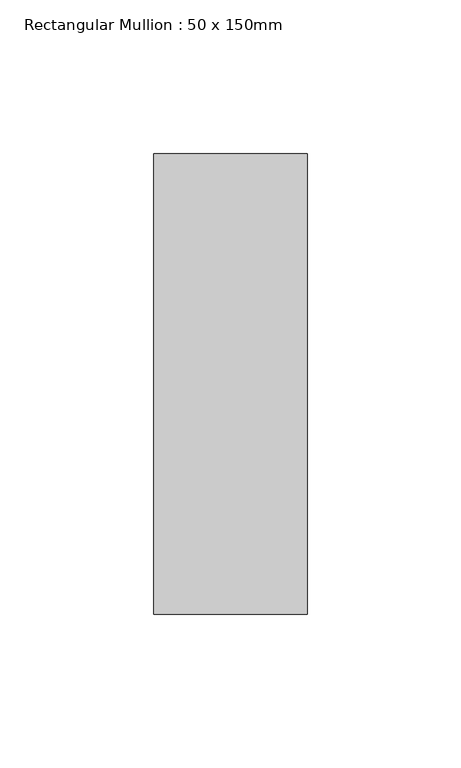
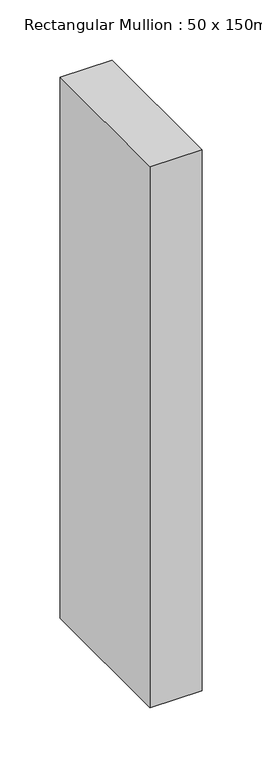
"""IFC4 building model written with IfcOpenShell, lengths in millimetres: member geometry, Rectangular Mullion : 50 x 150mm."""

from ifc_helpers import new_model, si_unit, frame, origin, place, context, project, spatial, polyline, outline, extrude, source, transform, mapped, element, save


def rectangular_mullion_50_x_150mm_5dbd0429(model_context):
    return source(origin(), model_context, "Body", "SweptSolid", [
        extrude(outline(polyline([(0.0, 75.0), (0.0, -75.0), (-50.0, -75.0), (-50.0, 75.0), (0.0, 75.0)])), frame((0.0, 0.0, -550.0), z_axis=(0.0, 0.0, 1.0), x_axis=(1.0, 0.0, 0.0)), (0.0, 0.0, 1.0), 550.0),
    ])


if __name__ == "__main__":
    model = new_model("IFC4")
    model_context = context("Model", 3, world=origin())
    ifc_project = project(units=[si_unit("LENGTHUNIT", "METRE", prefix="MILLI")], contexts=[model_context])
    site = spatial("IfcSite", under=ifc_project)
    building = spatial("IfcBuilding", under=site)
    placement = place(None, origin())
    rectangular_mullion_50_x_150mm_shape = rectangular_mullion_50_x_150mm_5dbd0429(model_context)
    element("IfcMember", 1, ObjectType="Rectangular Mullion : 50 x 150mm", at=placement, inside=building, context=model_context, shape_type="MappedRepresentation", body=[
        mapped(rectangular_mullion_50_x_150mm_shape, transform((0.0, 0.0, 0.0), x_axis=(1.0, 0.0, 0.0), y_axis=(0.0, 1.0, 0.0), z_axis=(0.0, 0.0, 1.0))),
    ])
    save(model, "model.ifc")

# Revit data of these elements
# Type "Rectangular Mullion : 50 x 150mm"
#   built-in parameter 1007304 = 0.492126 (stored number, unit not read)
#   built-in parameter 1007301 = 0.082021 (stored number, unit not read)
#   built-in parameter 1007300 = 0.082021 (stored number, unit not read)
# Element 1 (IfcMember, "Rectangular Mullion : 50 x 150mm")
#   Materials on its faces: "Aluminium"
# Materials
#   "Aluminium": class "Metal", colour RGB 247 247 247, transparency 0, Description = "Aluminium 6061", Cost = 0
